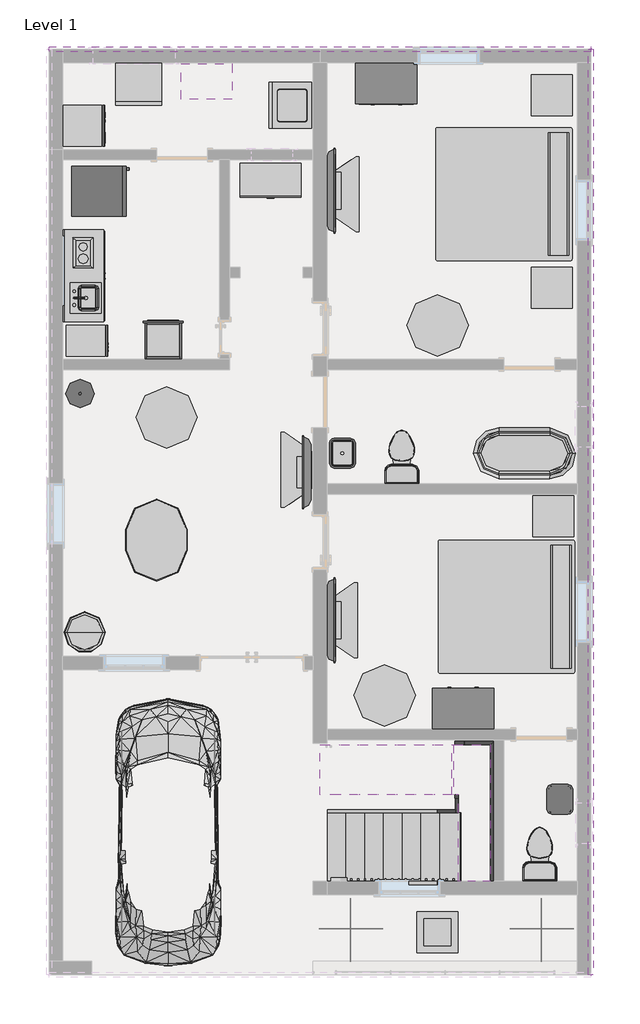
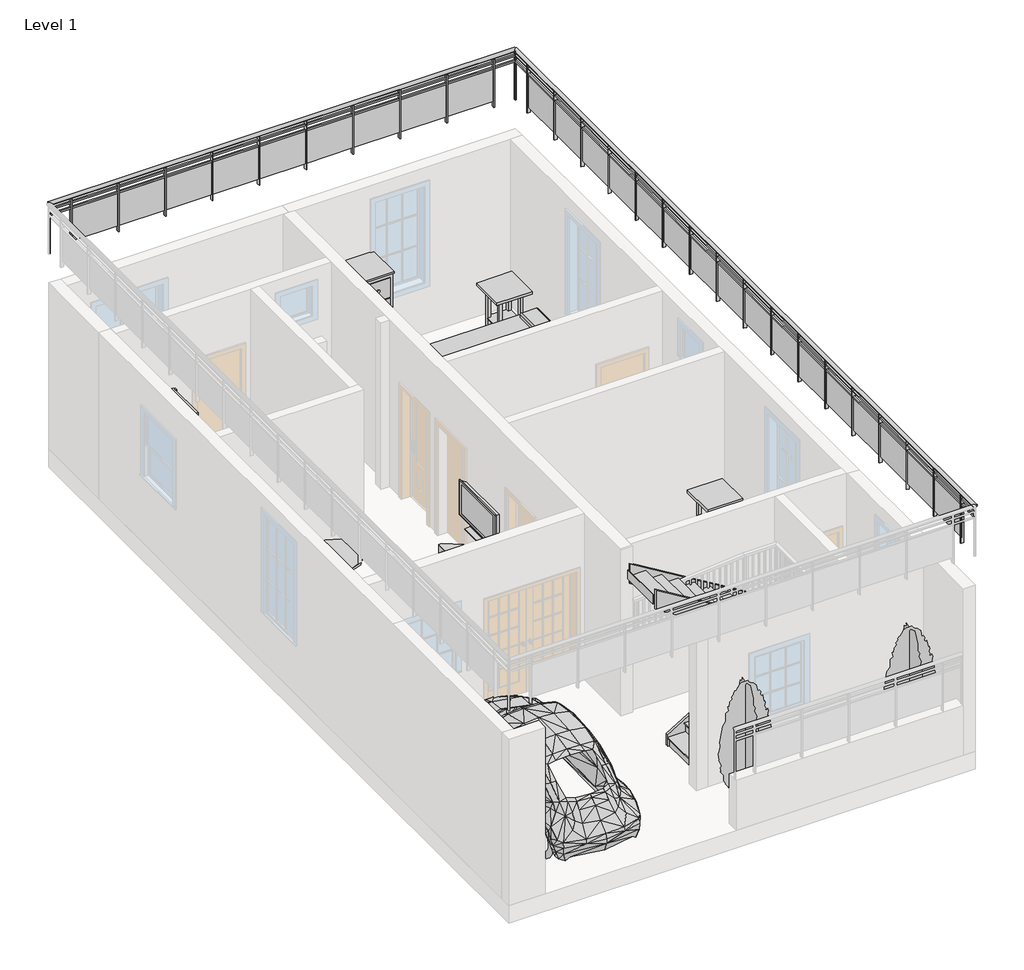
# One storey, part 3 of 3: 21 furniture elements, 9 proxies, 8 flow terminals, 8 members, 2 geographic elements, 2 railings, 2 stair flights, 1 slab.
# Revit data of these elements (continued)
# Type "RPC Tree - Conifer : Chinese Juniper - 7'" (continued)
#   built-in parameter 1005198 = "{2, 15},{39, RPC-16-FUM3-UUQ0-UBF0-N000-ST1L-LVER-AU},{1, 0},{1, 0},{2, 13},{1, 8},{5, Color},{1, 0},{1, 0},{3, 0.8},{3, 0.8},{3, 0.8},{1, 8},{7, BBoxMin},{1, 0},{1, 0},{1, 0},{1, 0},{1, 0},{1, 8},{7, BBoxMax},{1, 0},{1, 0},{1, 0},{1, 0},{1, 0},{2, 11},{9, RPCTypeId},{1, 0},{1, 0},{39, RPC-16-FUM3-UUQ0-UBF0-N000-ST1L-LVER-AU},{1, 6},{14, RPCPlantHeight},{1, 0},{1, 0},{1, 7},{2, 11},{7, keyword},{1, 0},{1, 0},{34, :RPCs:Trees [General]:Geometry:RPC},{2, 11},{8, category},{1, 0},{1, 0},{15, Trees [General]},{2, 11},{12, LocalizedUID},{1, 0},{1, 0},{15, Chinese Juniper},{2, 14},{6, Height},{1, 0},{1, 0},{1, 7},{1, 2},{16, Cast Reflections},{1, 0},{1, 0},{1, 0},{1, 2},{12, Cast Shadows},{1, 0},{1, 0},{1, 1},{1, 2},{9, Lock View},{1, 0},{1, 0},{1, 0},{1, 4},{5, ViewC},{1, 0},{1, 0},{1, 0},{21, assetlibrary_base.fbx},{1, 5},"
#   built-in parameter 1005195 = "RPC-16-FUM3-UUQ0-UBF0-N000-ST1L-LVER-AU"
#   Type Comments = "Chinese Juniper"
#   Assembly Code = "G2050500"
#   Height = 7' - 0"
#   Description = (empty or 0)
#   Default Elevation = 0
# Type "Glass Panel - Bottom Fill"
#   Assembly Code = "C2010400"
#   built-in parameter 1008612 = 0.0416667 (stored number, unit not read)
#   built-in parameter 1008611 = 0.0416667 (stored number, unit not read)
#   built-in parameter 1008609 = 0.333333 (stored number, unit not read)
#   built-in parameter 1008604 = 0.166667 (stored number, unit not read)
#   built-in parameter 1008603 = 0.166667 (stored number, unit not read)
#   Railing Height = 3' - 0"
#   built-in parameter 1008630 = 2
#   built-in parameter 1008610 = 2
#   built-in parameter 1008618 = Baluster - Square : 3/4"
# Element 1 (IfcBuildingElementProxy, "18\" x 24\" x 34 1/2\"")
#   Phase Created = New Construction
#   Materials on its faces: "Steel, Paint Finish, Ivory, Matte", "Plastic, Opaque Black"
# Element 2 (IfcBuildingElementProxy, "Cook Top-2 Unit : 12\" x 18\"")
#   Phase Created = New Construction
#   Materials on its faces: "Steel, Chrome Plated", "Steel, Polished"
# Element 3 (IfcBuildingElementProxy, "Dishwasher : 24\" x 24\" x 34\"")
#   Phase Created = New Construction
#   Materials on its faces: "Steel, Paint Finish, Ivory, Glossy", "Plastic, Opaque Black"
# Element 4 (IfcBuildingElementProxy, "Dryer : 27\" x 25\" x 35\"")
#   Phase Created = New Construction
#   Materials on its faces: "Steel, Paint Finish, Ivory, Glossy"
# Element 5 (IfcBuildingElementProxy, "Kitchenette - Small : 54\"")
#   Phase Created = New Construction
#   Materials on its faces: "Cabinets", "Cabinets - Handles"
# Element 6 (IfcBuildingElementProxy, "Oven Double-Built-in : 21 1/2\" x 39 1/4\" x 21\"")
#   Phase Created = New Construction
#   Materials on its faces: "Steel", "Metal - Stainless Steel, Polished", "Glass"
# Element 7 (IfcBuildingElementProxy, "RPC Beetle : RPC Beetle")
#   Phase Created = New Construction
# Element 8 (IfcBuildingElementProxy, "Refrigerator : 30\" x 32\" RH")
#   Phase Created = New Construction
#   Materials on its faces: "Steel, Paint Finish, Ivory, Glossy", "Steel, Chrome Plated"
# Element 9 (IfcBuildingElementProxy, "Washer : 27\" x 25\" x 35\"")
#   Phase Created = New Construction
#   Materials on its faces: "Steel, Paint Finish, Ivory, Matte"
# Element 10 (IfcFlowTerminal, "Sink Kitchen-Island : 18\" x 18\"")
#   Mark = "7"
#   Phase Created = New Construction
#   Materials on its faces: "Steel, Polished"
# Element 11 (IfcFlowTerminal, "Sink Kitchen-Single : 30\" x 21\"")
#   Mark = "8"
#   Phase Created = New Construction
#   Materials on its faces: "Steel, Polished"
# Element 12 (IfcFlowTerminal, "Sink Vanity-Round : 19\" x 19\"")
#   Mark = "9"
#   Phase Created = New Construction
#   Materials on its faces: "Porcelain, Linen", "Steel, Polished"
# Element 13 (IfcFlowTerminal, "Sink Vanity-Square : 20\" x 18\"")
#   Mark = "5"
#   Phase Created = New Construction
#   Materials on its faces: "Porcelain, Linen", "Steel, Polished"
# Element 14 (IfcFlowTerminal, "Sink Vanity-Square : 20\" x 18\"")
#   Mark = "6"
#   Phase Created = New Construction
#   Materials on its faces: "Porcelain, Linen", "Steel, Polished"
# Element 15 (IfcFlowTerminal, "Toilet-Domestic-3D : Toilet-Domestic-3D")
#   Mark = "1"
#   Phase Created = New Construction
#   Materials on its faces: "Porcelain, Linen", "Laminate, Linen, Matte"
# Element 16 (IfcFlowTerminal, "Toilet-Domestic-3D : Toilet-Domestic-3D")
#   Mark = "2"
#   Phase Created = New Construction
#   Materials on its faces: "Porcelain, Linen", "Laminate, Linen, Matte"
# Element 17 (IfcFlowTerminal, "Tub-Free Standing-3D : 30\" x 60\"")
#   Mark = "4"
#   Phase Created = New Construction
#   Materials on its faces: "Porcelain, Ivory"
# Elements 18, 19 (IfcFurniture, "Bed-Standard.0001 : King 78\" x 80\"")
#   Phase Created = New Construction
#   Materials on its faces: "Linen, White", "Steel, Chrome Plated"
# Element 20 (IfcFurniture, "Counter Top w Sink Hole : 24\" Depth")
#   Sink Opening Depth = 1' - 3"
#   Sink Location To Wall = 0' - 6"
#   Length = 4' - 6"
#   Sink Location = 1' - 2"
#   Sink Opening Width = 1' - 4"
#   Depth = 2' - 0"
#   Phase Created = New Construction
#   Materials on its faces: "Counter Top"
# Elements 21, 22 (IfcFurniture, "Dresser : 48\" x 72\" x 24\"")
#   Phase Created = New Construction
#   Materials on its faces: "Laminate, Ivory, Matte", "Cherry", "Laminate - Ivory, Glossy"
# Element 23 (IfcFurniture, "Storage Pedestal : 20\" x 36\" x 36\"")
#   Phase Created = New Construction
#   Materials on its faces: "Steel, Paint Finish, Ivory, Glossy", "Steel, Chrome Plated"
# Element 24 (IfcFurniture, "TV - Flat Screen : 42\"")
#   Stand = yes
#   Phase Created = New Construction
#   Materials on its faces: "TV - Black", "TV - Glass", "TV - Screen"
# Elements 25, 26 (IfcFurniture, "TV - Flat Screen : 50\"")
#   Stand = yes
#   Phase Created = New Construction
#   Materials on its faces: "TV - Black", "TV - Glass", "TV - Screen"
# Elements 27, 28, 29 (IfcFurniture, "TV Stand : TV Stand")
#   Phase Created = New Construction
#   Materials on its faces: "Melamine - Gray", "Glass - Shelves"
# Element 30 (IfcFurniture, "Table-Coffee : 24\" x 24\" x 24\"")
#   Phase Created = New Construction
#   Materials on its faces: "Glass - Clear, Grey"
# Element 31 (IfcFurniture, "Table-Dining Oval : 36\" x 72\"")
#   Phase Created = New Construction
#   Materials on its faces: "Steel, Chrome Plated", "Glass - Clear, Grey"
# Element 32 (IfcFurniture, "Table-Dining Round w Chairs : 36\" Diameter")
#   Phase Created = New Construction
#   Materials on its faces: "Pine", "Laminate, Linen, Matte"
# Elements 33, 34 (IfcFurniture, "Table-Ellipse : 72\" x 36\"")
#   Phase Created = New Construction
#   Materials on its faces: "Birch", "Laminate - Black"
# Elements 35, 36, 37 (IfcFurniture, "Table-Night Stand : 24\" x 24\" x 30\"")
#   Phase Created = New Construction
#   Materials on its faces: "Birch", "Laminate, Ivory, Matte"
# Element 38 (IfcFurniture, "Table-Round : 36\" Diameter")
#   Phase Created = New Construction
#   Materials on its faces: "Steel, Chrome Plated", "Birch"
# Elements 39, 40 (IfcGeographicElement, "RPC Tree - Conifer : Chinese Juniper - 7'")
#   Phase Created = New Construction
# Elements 41, 42, 43, 44, 45, 46, 47, 48 (IfcMember, "Stringer - 2\" Width")
#   Phase Created = New Construction
# Elements 49, 50 (IfcRailing, "Glass Panel - Bottom Fill")
#   built-in parameter 1008621 = 11.75 (stored number, unit not read)
#   Phase Created = New Construction
#   Materials on its faces: "Glass"
# Element 51 (IfcSlab, "Non-Monolithic Landing")
#   Phase Created = New Construction
# Elements 52, 53 (IfcStairFlight, "2\" Tread 1\" Nosing 1/4\" Riser")
#   Phase Created = New Construction
# Materials
#   "Plastic, Opaque Black": class "Plastic", colour RGB 0 0 0, transparency 0.7, Description = "Plastic, generic, opaque black", Cost = 0
#   "Steel, Paint Finish, Ivory, Matte": class "Metal", colour RGB 247 247 239, transparency 0, Description = "Steel, paint finish, ivory, matte", Cost = 0
#   "Steel, Chrome Plated": class "Metal", colour RGB 17 17 17, transparency 0, Description = "Chromiuim plated steel", Cost = 0
#   "Steel, Polished": class "Metal", colour RGB 57 57 57, transparency 0, Description = "Polished steel", Cost = 0
#   "Steel, Paint Finish, Ivory, Glossy": class "Metal", colour RGB 247 247 239, transparency 0, Description = "Steel, paint finish, ivory, glossy", Cost = 0
#   "Cabinets": colour RGB 249 249 249, transparency 0
#   "Cabinets - Handles": class "Metal", colour RGB 57 57 57, transparency 0
#   "Metal - Stainless Steel, Polished": class "Metal", colour RGB 216 216 216, transparency 0
#   "Porcelain, Linen": class "Ceramic", colour RGB 249 239 230, transparency 0, Description = "Porcelain, linen", Cost = 0
#   "Laminate, Linen, Matte": class "Plastic", colour RGB 249 239 230, transparency 0, Description = "Plastic Laminate - Linen, Matte", Cost = 0
#   "Porcelain, Ivory": class "Ceramic", colour RGB 247 247 239, transparency 0, Description = "Porcelain, ivory", Cost = 0
#   "Linen, White": class "Textile", colour RGB 247 247 239, transparency 0, Description = "Linen, white", Cost = 0
#   "Laminate - Ivory, Glossy": colour RGB 247 247 239, transparency 0
#   "Laminate, Ivory, Matte": class "Plastic", colour RGB 247 247 239, transparency 0, Description = "Plastic Laminate - Ivory, Matte", Cost = 0
#   "Cherry": class "Wood", colour RGB 226 177 128, transparency 0, Description = "Prunus Serotina", Cost = 0
#   "Melamine - Gray": class "Wood", colour RGB 49 49 49, transparency 0
#   "Glass - Clear, Grey": class "Glass", colour RGB 252 255 255, transparency 0.64
#   "Pine": class "Wood", colour RGB 223 192 134, transparency 0, Description = "Pinus Echinata", Cost = 0
#   "Birch": class "Wood", colour RGB 224 178 126, transparency 0, Description = "Betula Alleghaniensis", Cost = 0
#   "Laminate - Black": colour RGB 0 0 0, transparency 0
#   "Steel": class "Metal", colour RGB 247 247 247, transparency 0, Description = "Steel, mill finish", Cost = 0
#   "Glass": class "Glass", colour RGB 0 128 192, transparency 0.75, Description = "Soda Lime Glass", Cost = 0
#   "Counter Top": class "Wood", colour RGB 226 177 128, transparency 0
#   "TV - Black": colour RGB 49 49 49, transparency 0
#   "TV - Glass": colour RGB 157 157 157, transparency 0.9
#   "TV - Screen": colour RGB 0 0 0, transparency 0
#   "Glass - Shelves": class "Glass", colour RGB 167 167 167, transparency 0.9
